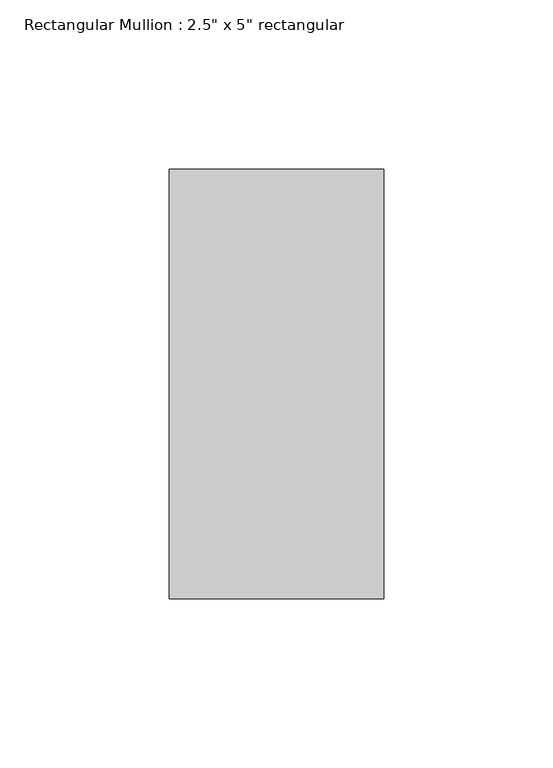
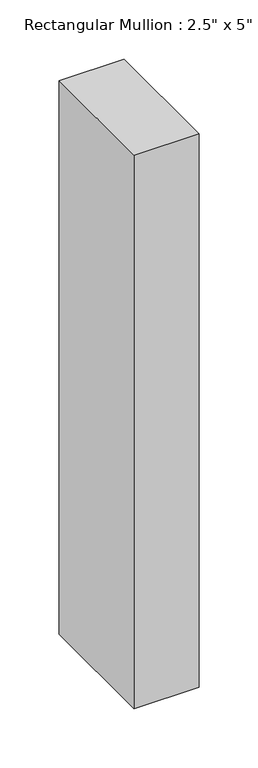
"""IFC4 building model written with IfcOpenShell, lengths in millimetres: member geometry."""

from ifc_helpers import new_model, si_unit, frame, origin, place, context, project, spatial, polyline, outline, extrude, source, transform, mapped, element, save


def member_c8189573(model_context):
    return source(origin(), model_context, "Body", "SweptSolid", [
        extrude(outline(polyline([(0.0, 63.5), (0.0, -63.5), (-63.5, -63.5), (-63.5, 63.5), (0.0, 63.5)])), frame((0.0, 0.0, -571.5), z_axis=(0.0, 0.0, 1.0), x_axis=(1.0, 0.0, 0.0)), (0.0, 0.0, 1.0), 571.5),
    ])


if __name__ == "__main__":
    model = new_model("IFC4")
    model_context = context("Model", 3, world=origin())
    ifc_project = project(units=[si_unit("LENGTHUNIT", "METRE", prefix="MILLI")], contexts=[model_context])
    site = spatial("IfcSite", under=ifc_project)
    building = spatial("IfcBuilding", under=site)
    placement = place(None, origin())
    member_shape = member_c8189573(model_context)
    element("IfcMember", 1, ObjectType="Rectangular Mullion : 2.5\" x 5\" rectangular", at=placement, inside=building, context=model_context, shape_type="MappedRepresentation", body=[
        mapped(member_shape, transform((0.0, 0.0, 0.0), x_axis=(1.0, 0.0, 0.0), y_axis=(0.0, 1.0, 0.0), z_axis=(0.0, 0.0, 1.0))),
    ])
    save(model, "model.ifc")

# Revit data of these elements
# Type "Rectangular Mullion : 2.5\" x 5\" rectangular"
#   built-in parameter 1007304 = 0.416667 (stored number, unit not read)
#   built-in parameter 1007301 = 0.104167 (stored number, unit not read)
#   built-in parameter 1007300 = 0.104167 (stored number, unit not read)
# Element 1 (IfcMember, "Rectangular Mullion : 2.5\" x 5\" rectangular")
#   Materials on its faces: "Aluminum"
# Materials
#   "Aluminum": class "Metal", colour RGB 247 247 247, transparency 0, Description = "Aluminum 6061", Cost = 0
